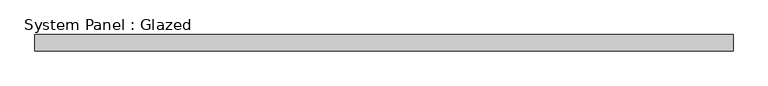
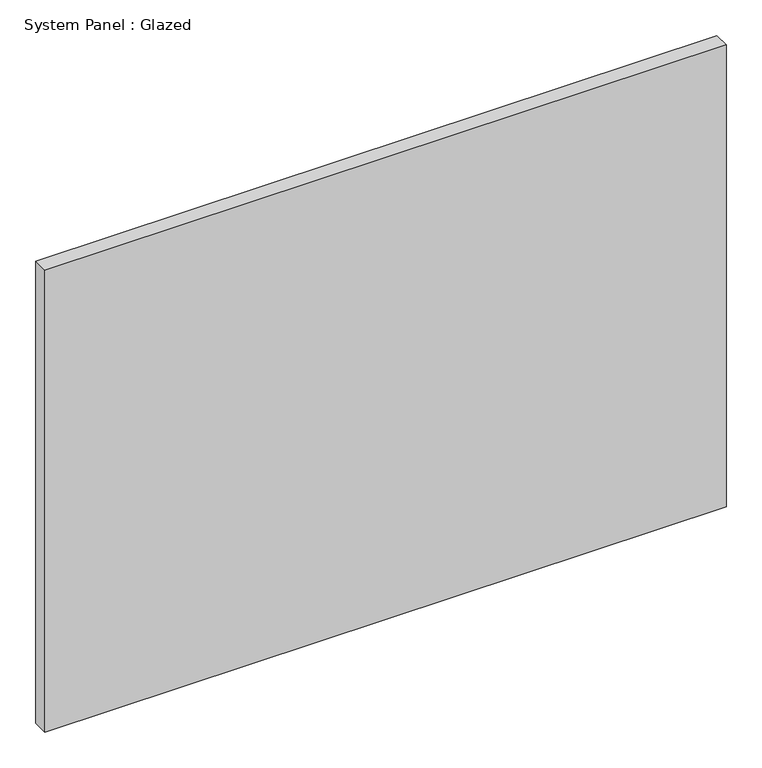
"""IFC4 building model written with IfcOpenShell, lengths in millimetres: plate geometry, System Panel : Glazed."""

from ifc_helpers import new_model, si_unit, origin, origin_with_axes, place, context, project, spatial, polyline, outline, extrude, source, transform, mapped, element, save


def system_panel_glazed_3f576ca0(model_context):
    return source(origin(), model_context, "Body", "SweptSolid", [
        extrude(outline(polyline([(549.275, 19.05), (-549.275, 19.05), (-549.275, 44.45), (549.275, 44.45), (549.275, 19.05)])), origin_with_axes(), (0.0, 0.0, 1.0), 787.4),
    ])


if __name__ == "__main__":
    model = new_model("IFC4")
    model_context = context("Model", 3, world=origin())
    ifc_project = project(units=[si_unit("LENGTHUNIT", "METRE", prefix="MILLI")], contexts=[model_context])
    site = spatial("IfcSite", under=ifc_project)
    building = spatial("IfcBuilding", under=site)
    placement = place(None, origin())
    system_panel_glazed_shape = system_panel_glazed_3f576ca0(model_context)
    element("IfcPlate", 1, ObjectType="System Panel : Glazed", at=placement, inside=building, context=model_context, shape_type="MappedRepresentation", body=[
        mapped(system_panel_glazed_shape, transform((0.0, 0.0, 0.0), x_axis=(1.0, 0.0, 0.0), y_axis=(0.0, 1.0, 0.0), z_axis=(0.0, 0.0, 1.0))),
    ])
    save(model, "model.ifc")

# Revit data of these elements
# Type "System Panel : Glazed"
#   Construction Type Id = "GSP4R"
#   Analytic Construction = "1/8 in Pilkington single glazing"
#   Visual Light Transmittance = 0.9
#   Solar Heat Gain Coefficient = 0.86
#   Heat Transfer Coefficient (U) = 1.18115 BTU/(h·ft²·°F)
# Element 1 (IfcPlate, "System Panel : Glazed")
#   Materials on its faces: "Glass"
# Materials
#   "Glass": class "Glass", colour RGB 0 128 192, transparency 0.75, Description = "Soda Lime Glass", Cost = 0
